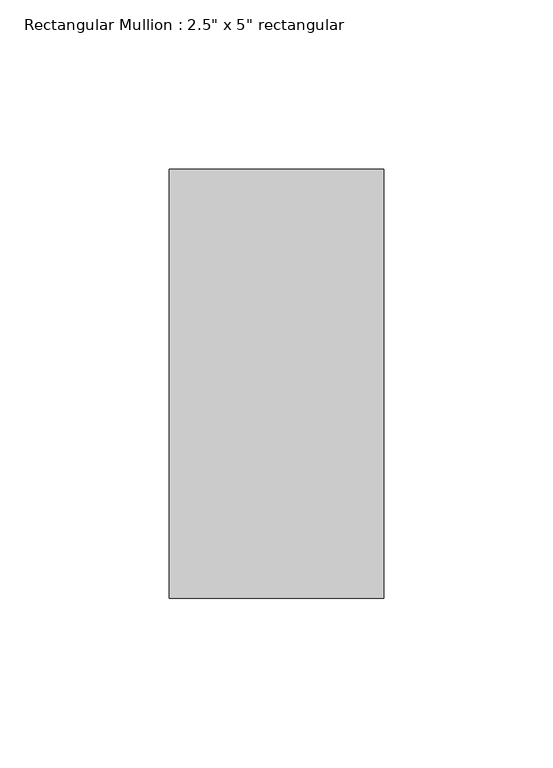
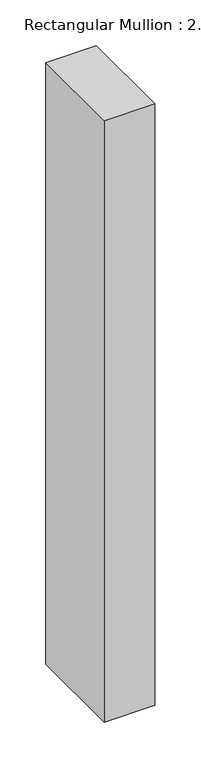
"""IFC4 building model written with IfcOpenShell, lengths in millimetres: member geometry."""

from ifc_helpers import new_model, si_unit, frame, origin, place, context, project, spatial, polyline, outline, extrude, source, transform, mapped, element, save


def member_cfa99961(model_context):
    return source(origin(), model_context, "Body", "SweptSolid", [
        extrude(outline(polyline([(31.75, 63.5), (31.75, -63.5), (-31.75, -63.5), (-31.75, 63.5), (31.75, 63.5)])), frame((0.0, 0.0, -800.1), z_axis=(0.0, 0.0, 1.0), x_axis=(1.0, 0.0, 0.0)), (0.0, 0.0, 1.0), 800.1),
    ])


if __name__ == "__main__":
    model = new_model("IFC4")
    model_context = context("Model", 3, world=origin())
    ifc_project = project(units=[si_unit("LENGTHUNIT", "METRE", prefix="MILLI")], contexts=[model_context])
    site = spatial("IfcSite", under=ifc_project)
    building = spatial("IfcBuilding", under=site)
    placement = place(None, origin())
    member_shape = member_cfa99961(model_context)
    element("IfcMember", 1, ObjectType="Rectangular Mullion : 2.5\" x 5\" rectangular", at=placement, inside=building, context=model_context, shape_type="MappedRepresentation", body=[
        mapped(member_shape, transform((0.0, 0.0, 0.0), x_axis=(1.0, 0.0, 0.0), y_axis=(0.0, 1.0, 0.0), z_axis=(0.0, 0.0, 1.0))),
    ])
    save(model, "model.ifc")

# Revit data of these elements
# Type "Rectangular Mullion : 2.5\" x 5\" rectangular"
#   built-in parameter 1007304 = 0.416667 (stored number, unit not read)
#   built-in parameter 1007301 = 0.104167 (stored number, unit not read)
#   built-in parameter 1007300 = 0.104167 (stored number, unit not read)
# Element 1 (IfcMember, "Rectangular Mullion : 2.5\" x 5\" rectangular")
#   Materials on its faces: "Aluminum"
# Materials
#   "Aluminum": class "Metal", colour RGB 247 247 247, transparency 0, Description = "Aluminum 6061", Cost = 0
